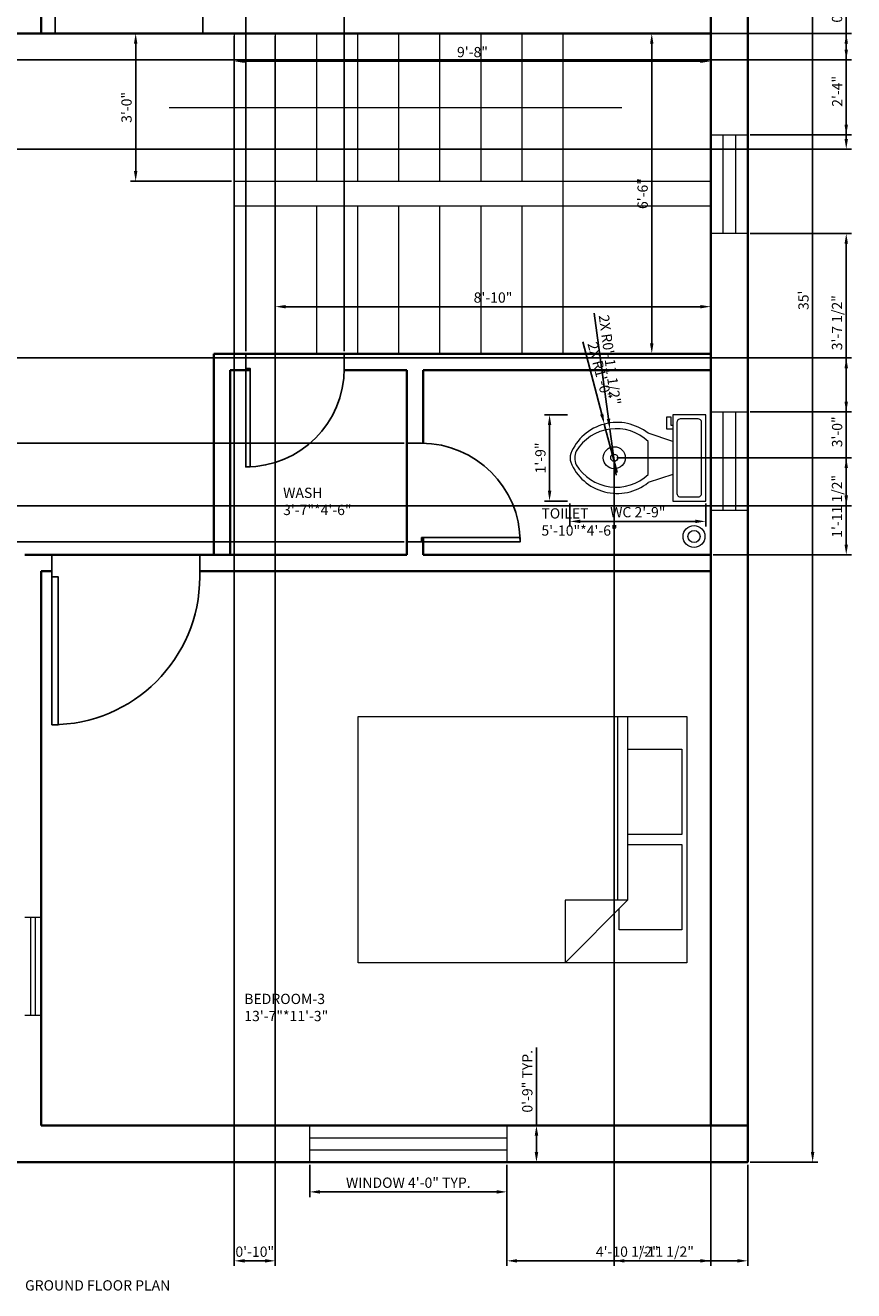
# Model space of a CAD drawing. Units: inches. Extents: x 2655 to 3059, y 1617 to 2098.
# Tile 2 of 3: x 2857 to 3059, y 1617 to 1926. Entities that reach past the tile are written whole.
import ezdxf

# ---------------------------------------------------------------- set-up
doc = ezdxf.new("R2010")
doc.units = ezdxf.units.IN
for name, color, linetype, lineweight in [('A-ANNO-DIMS', 2, 'Continuous', 18), ('A-ANNO-TEXT', 7, 'Continuous', 18), ('A-AREA-IDEN', 7, 'Continuous', 18), ('A-DOOR', 3, 'Continuous', 25), ('A-FLOR-FIXT', 9, 'Continuous', 18), ('A-FLOR-STRS', 7, 'Continuous', 20), ('A-FURN', 8, 'Continuous', 18), ('A-GLAZ', 4, 'Continuous', 18), ('A-WALL', 7, 'Continuous', 35)]:
    doc.layers.add(name, color=color, linetype=linetype, lineweight=lineweight)
doc.styles.get("Standard").update_dxf_attribs({"font": 'arial.ttf'})
doc.dimstyles.new('ISO-25', dxfattribs={"dimtxt": 2.5, "dimasz": 2.5, "dimexe": 1.25, "dimexo": 0.625, "dimtad": 1, "dimdec": 1, "dimlunit": 3, "dimtxsty": 'Standard', "dimcen": 2.5, "dimadec": 0, "dimazin": 0, "dimtfac": 1, "dimtdec": 1, "dimtmove": 0, "dimatfit": 3, "dimfxl": 1, "dimarcsym": 0})

# ---------------------------------------------------------------- blocks, each defined once
blk = doc.blocks.new('*D1')
at = {"layer": 'A-ANNO-DIMS', "color": 0, "lineweight": -2, "transparency": 16777216}
for p, q in [((2907.77, 1923.14), (2907.77, 1915.77)), ((3023.77, 1923.14), (3023.77, 1915.77)), ((2910.27, 1917.02), (3021.27, 1917.02))]:
    blk.add_line(p, q, dxfattribs=at)
at = {"layer": 'A-ANNO-DIMS', "color": 0, "transparency": 16777216}
for points in [[(2910.27, 1917.43), (2910.27, 1916.6), (2907.77, 1917.02)], [(3021.27, 1917.43), (3021.27, 1916.6), (3023.77, 1917.02)]]:
    blk.add_solid(points, dxfattribs=at)
at = {"layer": 'Defpoints', "color": 0, "transparency": 16777216}
for p in [(2907.77, 1923.77), (3023.77, 1923.77), (3023.77, 1917.02)]:
    blk.add_point(p, dxfattribs=at)
at = {"layer": 'A-ANNO-DIMS', "color": 0, "transparency": 16777216, "insert": (2965.77, 1918.92), "char_height": 2.5, "attachment_point": 5}
blk.add_mtext('9\'-8"', dxfattribs=at)
blk = doc.blocks.new('*D2')
at = {"layer": 'A-ANNO-DIMS', "color": 0, "lineweight": -2, "transparency": 16777216}
for p, q in [((2917.77, 1846.39), (2917.77, 1858.47)), ((2920.27, 1857.22), (3021.27, 1857.22)), ((3023.77, 1846.39), (3023.77, 1858.47))]:
    blk.add_line(p, q, dxfattribs=at)
at = {"layer": 'A-ANNO-DIMS', "color": 0, "transparency": 16777216}
for points in [[(2920.27, 1857.63), (2920.27, 1856.8), (2917.77, 1857.22)], [(3021.27, 1857.63), (3021.27, 1856.8), (3023.77, 1857.22)]]:
    blk.add_solid(points, dxfattribs=at)
at = {"layer": 'Defpoints', "color": 0, "transparency": 16777216}
for p in [(3023.77, 1857.22), (2917.77, 1845.77), (3023.77, 1845.77)]:
    blk.add_point(p, dxfattribs=at)
at = {"layer": 'A-ANNO-DIMS', "color": 0, "transparency": 16777216, "insert": (2970.77, 1859.12), "char_height": 2.5, "attachment_point": 5}
blk.add_mtext('8\'-10"', dxfattribs=at)
blk = doc.blocks.new('*D3')
at = {"layer": 'A-ANNO-DIMS', "color": 0, "lineweight": -2, "transparency": 16777216}
for p, q in [((3023.14, 1923.77), (3008.17, 1923.77)), ((3009.42, 1921.27), (3009.42, 1848.27)), ((3023.14, 1845.77), (3008.17, 1845.77))]:
    blk.add_line(p, q, dxfattribs=at)
at = {"layer": 'A-ANNO-DIMS', "color": 0, "transparency": 16777216}
for points in [[(3009, 1921.27), (3009.84, 1921.27), (3009.42, 1923.77)], [(3009, 1848.27), (3009.84, 1848.27), (3009.42, 1845.77)]]:
    blk.add_solid(points, dxfattribs=at)
at = {"layer": 'Defpoints', "color": 0, "transparency": 16777216}
for p in [(3023.77, 1923.77), (3009.42, 1845.77), (3023.77, 1845.77)]:
    blk.add_point(p, dxfattribs=at)
at = {"layer": 'A-ANNO-DIMS', "color": 0, "transparency": 16777216, "insert": (3007.52, 1884.77), "char_height": 2.5, "attachment_point": 5, "rotation": 90}
blk.add_mtext('6\'-6"', dxfattribs=at)
blk = doc.blocks.new('*U5')
for p, q in [((0, 0), (0, -6)), ((40, 0), (40, -6))]:
    blk.add_line(p, q)
blk.add_lwpolyline([(0, 0), (0, 40), (1.75, 40), (1.75, 0)], close=True)
blk.add_arc((0, 0), 40, 0, 90)
blk = doc.blocks.new('Bed - Queen')
for p, q in [((0, -80.00003), (0, 0)), ((0, 0), (59.99999, 0)), ((59.99999, 0), (59.99999, -80.00003)), ((7.99999, -1.2), (28.79998, -1.2)), ((7.99999, -14.4), (7.99999, -1.2)), ((28.79998, -1.2), (28.79998, -14.4)), ((31.19999, -1.2), (51.99999, -1.2)), ((31.19999, -14.4), (31.19999, -1.2)), ((51.99999, -1.2), (51.99999, -16.4)), ((0, -14.4), (44.8, -14.4)), ((59.99999, -29.6), (44.8, -14.4)), ((44.8, -14.4), (44.8, -29.6)), ((44.8, -16.8), (0, -16.8)), ((51.99999, -16.4), (46.79936, -16.4)), ((44.8, -29.6), (59.99999, -29.6)), ((59.99999, -80.00003), (0, -80.00003))]:
    blk.add_line(p, q)
blk = doc.blocks.new('Toilet - top')
for p, q in [((9.5, -6), (9.5, -2)), ((-10, -8.5), (-8, -8.5)), ((-10, -9.5), (-10, -8.5)), ((-8, -8.5), (-8, -8)), ((-7, -8), (-7, -9.5)), ((-4, -8), (-6, -14)), ((4, -8), (6, -14)), ((-7, -9.5), (-10, -9.5)), ((4, -14), (-4, -14))]:
    blk.add_line(p, q)
blk.add_lwpolyline([(10.5, -8), (10.5, 0), (-10.5, 0), (-10.5, -8)], close=True)
for points in [[(-9.5, -2), (-9.5, -6)], [(8.5, -1), (-8.5, -1)], [(-8.5, -7), (8.5, -7)]]:
    blk.add_lwpolyline(points)
for centre, radius, start, end in [((-8.62, -1.88), 0.884, 81.8699, 188.1301), ((8.62, -1.88), 0.884, 351.8699, 98.1301), ((-8.62, -6.12), 0.884, 171.8699, 278.1301), ((8.62, -6.12), 0.884, 261.8699, 8.1301), ((3.52, -21.58), 12.17, 141.4691, 247.9714), ((4.2, -21.82), 11.33, 136.3677, 238.9468), ((-3.52, -21.58), 12.17, 292.0284, 38.5307), ((-4.2, -21.82), 11.33, 301.053, 43.6321), ((0, -27.88), 4, 245.7318, 294.2682), ((0, -29), 4, 254.8605, 285.1395)]:
    blk.add_arc(centre, radius, start, end)
blk = doc.blocks.new('*D10')
at = {"layer": 'A-ANNO-DIMS', "color": 0, "lineweight": -2, "transparency": 16777216}
for p, q in [((3033.39, 2068.77), (3049.84, 2068.77)), ((3048.59, 2066.27), (3048.59, 1651.27)), ((3033.39, 1648.77), (3049.84, 1648.77))]:
    blk.add_line(p, q, dxfattribs=at)
at = {"layer": 'A-ANNO-DIMS', "color": 0, "transparency": 16777216}
for points in [[(3048.17, 2066.27), (3049, 2066.27), (3048.59, 2068.77)], [(3048.17, 1651.27), (3049, 1651.27), (3048.59, 1648.77)]]:
    blk.add_solid(points, dxfattribs=at)
at = {"layer": 'Defpoints', "color": 0, "transparency": 16777216}
for p in [(3032.77, 2068.77), (3032.77, 1648.77), (3048.59, 1648.77)]:
    blk.add_point(p, dxfattribs=at)
at = {"layer": 'A-ANNO-DIMS', "color": 0, "transparency": 16777216, "insert": (3046.68, 1858.77), "char_height": 2.5, "attachment_point": 5, "rotation": 90}
blk.add_mtext("35'", dxfattribs=at)
blk = doc.blocks.new('WIN-48x9')
for p, q in [((0, 9), (48, 9)), ((0, 0), (0, 9)), ((48, 9), (48, 0)), ((0, 6), (48, 6)), ((48, 3), (0, 3)), ((48, 0), (0, 0))]:
    blk.add_line(p, q)
blk = doc.blocks.new('WIN-24x9')
for p, q in [((0, 0), (0, 24)), ((0, 24), (9, 24)), ((3, 0), (3, 24)), ((6, 24), (6, 0)), ((9, 24), (9, 0)), ((9, 0), (0, 0))]:
    blk.add_line(p, q)
blk = doc.blocks.new('*D13')
at = {"layer": 'A-ANNO-DIMS', "color": 0, "lineweight": -2, "transparency": 16777216}
for p, q in [((2926.15, 1648.14), (2926.15, 1640.32)), ((2974.15, 1648.14), (2974.15, 1640.32)), ((2928.65, 1641.57), (2971.65, 1641.57))]:
    blk.add_line(p, q, dxfattribs=at)
at = {"layer": 'A-ANNO-DIMS', "color": 0, "transparency": 16777216}
for points in [[(2928.65, 1641.98), (2928.65, 1641.15), (2926.15, 1641.57)], [(2971.65, 1641.98), (2971.65, 1641.15), (2974.15, 1641.57)]]:
    blk.add_solid(points, dxfattribs=at)
at = {"layer": 'Defpoints', "color": 0, "transparency": 16777216}
for p in [(2926.15, 1648.77), (2974.15, 1648.77), (2974.15, 1641.57)]:
    blk.add_point(p, dxfattribs=at)
at = {"layer": 'A-ANNO-DIMS', "color": 0, "transparency": 16777216, "insert": (2950.15, 1643.48), "char_height": 2.5, "attachment_point": 5}
blk.add_mtext('WINDOW 4\'-0" TYP.', dxfattribs=at)
blk = doc.blocks.new('*D14')
at = {"layer": 'A-ANNO-DIMS', "color": 0, "lineweight": -2, "transparency": 16777216}
for p, q in [((2981.35, 1657.77), (2981.35, 1676.76)), ((2974.78, 1657.77), (2982.6, 1657.77)), ((2981.35, 1651.27), (2981.35, 1655.27)), ((2974.78, 1648.77), (2982.6, 1648.77))]:
    blk.add_line(p, q, dxfattribs=at)
at = {"layer": 'A-ANNO-DIMS', "color": 0, "transparency": 16777216}
for points in [[(2980.93, 1655.27), (2981.77, 1655.27), (2981.35, 1657.77)], [(2980.93, 1651.27), (2981.77, 1651.27), (2981.35, 1648.77)]]:
    blk.add_solid(points, dxfattribs=at)
at = {"layer": 'Defpoints', "color": 0, "transparency": 16777216}
for p in [(2974.15, 1657.77), (2981.35, 1657.77), (2974.15, 1648.77)]:
    blk.add_point(p, dxfattribs=at)
at = {"layer": 'A-ANNO-DIMS', "color": 0, "transparency": 16777216, "insert": (2979.45, 1668.51), "char_height": 2.5, "attachment_point": 5, "rotation": 90}
blk.add_mtext('0\'-9" TYP.', dxfattribs=at)
blk = doc.blocks.new('*D19')
at = {"layer": 'A-ANNO-DIMS', "color": 0, "lineweight": -2, "transparency": 16777216}
for p, q in [((2989.5, 1809.25), (2989.5, 1803.66)), ((3022.55, 1809.25), (3022.55, 1803.66)), ((2992, 1804.91), (3020.05, 1804.91))]:
    blk.add_line(p, q, dxfattribs=at)
at = {"layer": 'A-ANNO-DIMS', "color": 0, "transparency": 16777216}
for points in [[(2992, 1805.33), (2992, 1804.5), (2989.5, 1804.91)], [(3020.05, 1805.33), (3020.05, 1804.5), (3022.55, 1804.91)]]:
    blk.add_solid(points, dxfattribs=at)
at = {"layer": 'Defpoints', "color": 0, "transparency": 16777216}
for p in [(2989.5, 1809.87), (3022.55, 1809.87), (3022.55, 1804.91)]:
    blk.add_point(p, dxfattribs=at)
at = {"layer": 'A-ANNO-DIMS', "color": 0, "transparency": 16777216, "insert": (3006.02, 1806.83), "char_height": 2.5, "attachment_point": 5}
blk.add_mtext('WC 2\'-9"', dxfattribs=at)
blk = doc.blocks.new('*D20')
at = {"layer": 'A-ANNO-DIMS', "color": 0, "lineweight": -2, "transparency": 16777216}
for p, q in [((2988.88, 1830.87), (2983.29, 1830.87)), ((2984.54, 1828.37), (2984.54, 1812.37)), ((2988.88, 1809.87), (2983.29, 1809.87))]:
    blk.add_line(p, q, dxfattribs=at)
at = {"layer": 'A-ANNO-DIMS', "color": 0, "transparency": 16777216}
for points in [[(2984.13, 1828.37), (2984.96, 1828.37), (2984.54, 1830.87)], [(2984.13, 1812.37), (2984.96, 1812.37), (2984.54, 1809.87)]]:
    blk.add_solid(points, dxfattribs=at)
at = {"layer": 'Defpoints', "color": 0, "transparency": 16777216}
for p in [(2989.5, 1830.87), (2984.54, 1809.87), (2989.5, 1809.87)]:
    blk.add_point(p, dxfattribs=at)
at = {"layer": 'A-ANNO-DIMS', "color": 0, "transparency": 16777216, "insert": (2982.64, 1820.37), "char_height": 2.5, "attachment_point": 5, "rotation": 90}
blk.add_mtext('1\'-9"', dxfattribs=at)
blk = doc.blocks.new('*D27')
at = {"layer": 'A-ANNO-DIMS', "color": 0, "lineweight": -2, "transparency": 16777216}
for p, q in [((3033.39, 1985.21), (3058.02, 1985.21)), ((3056.77, 1982.71), (3056.77, 1901.56)), ((3033.39, 1899.06), (3058.02, 1899.06))]:
    blk.add_line(p, q, dxfattribs=at)
at = {"layer": 'A-ANNO-DIMS', "color": 0, "transparency": 16777216}
for points in [[(3056.35, 1982.71), (3057.19, 1982.71), (3056.77, 1985.21)], [(3056.35, 1901.56), (3057.19, 1901.56), (3056.77, 1899.06)]]:
    blk.add_solid(points, dxfattribs=at)
at = {"layer": 'Defpoints', "color": 0, "transparency": 16777216}
for p in [(3032.77, 1985.21), (3032.77, 1899.06), (3056.77, 1899.06)]:
    blk.add_point(p, dxfattribs=at)
at = {"layer": 'A-ANNO-DIMS', "color": 0, "transparency": 16777216, "insert": (3054.89, 1942.13), "char_height": 2.5, "attachment_point": 5, "rotation": 90}
blk.add_mtext('7\'-2"', dxfattribs=at)
blk = doc.blocks.new('*D28')
at = {"layer": 'A-ANNO-DIMS', "color": 0, "lineweight": -2, "transparency": 16777216}
for p, q in [((3033.39, 1875.06), (3058.02, 1875.06)), ((3056.77, 1872.56), (3056.77, 1834.08)), ((3033.39, 1831.58), (3058.02, 1831.58))]:
    blk.add_line(p, q, dxfattribs=at)
at = {"layer": 'A-ANNO-DIMS', "color": 0, "transparency": 16777216}
for points in [[(3056.35, 1872.56), (3057.19, 1872.56), (3056.77, 1875.06)], [(3056.35, 1834.08), (3057.19, 1834.08), (3056.77, 1831.58)]]:
    blk.add_solid(points, dxfattribs=at)
at = {"layer": 'Defpoints', "color": 0, "transparency": 16777216}
for p in [(3032.77, 1875.06), (3032.77, 1831.58), (3056.77, 1831.58)]:
    blk.add_point(p, dxfattribs=at)
at = {"layer": 'A-ANNO-DIMS', "color": 0, "transparency": 16777216, "insert": (3054.85, 1853.32), "char_height": 2.5, "attachment_point": 5, "rotation": 90}
blk.add_mtext('3\'-7 1/2"', dxfattribs=at)
blk = doc.blocks.new('*D29')
at = {"layer": 'A-ANNO-DIMS', "color": 0, "lineweight": -2, "transparency": 16777216}
for p, q in [((2974.15, 1648.14), (2974.15, 1623.52)), ((3032.77, 1648.14), (3032.77, 1623.52)), ((3030.27, 1624.77), (2976.65, 1624.77))]:
    blk.add_line(p, q, dxfattribs=at)
at = {"layer": 'A-ANNO-DIMS', "color": 0, "transparency": 16777216}
for points in [[(2976.65, 1625.18), (2976.65, 1624.35), (2974.15, 1624.77)], [(3030.27, 1625.18), (3030.27, 1624.35), (3032.77, 1624.77)]]:
    blk.add_solid(points, dxfattribs=at)
at = {"layer": 'Defpoints', "color": 0, "transparency": 16777216}
for p in [(2974.15, 1648.77), (3032.77, 1648.77), (2974.15, 1624.77)]:
    blk.add_point(p, dxfattribs=at)
at = {"layer": 'A-ANNO-DIMS', "color": 0, "transparency": 16777216, "insert": (3003.46, 1626.68), "char_height": 2.5, "attachment_point": 5}
blk.add_mtext('4\'-10 1/2"', dxfattribs=at)
blk = doc.blocks.new('*D37')
at = {"layer": 'A-ANNO-DIMS', "color": 0, "lineweight": -2, "transparency": 16777216}
for p, q in [((2907.77, 1923.14), (2907.77, 1623.52)), ((2917.77, 1923.14), (2917.77, 1623.52)), ((2910.27, 1624.77), (2915.27, 1624.77))]:
    blk.add_line(p, q, dxfattribs=at)
at = {"layer": 'A-ANNO-DIMS', "color": 0, "transparency": 16777216}
for points in [[(2910.27, 1625.18), (2910.27, 1624.35), (2907.77, 1624.77)], [(2915.27, 1625.18), (2915.27, 1624.35), (2917.77, 1624.77)]]:
    blk.add_solid(points, dxfattribs=at)
at = {"layer": 'Defpoints', "color": 0, "transparency": 16777216}
for p in [(2907.77, 1923.77), (2917.77, 1923.77), (2917.77, 1624.77)]:
    blk.add_point(p, dxfattribs=at)
at = {"layer": 'A-ANNO-DIMS', "color": 0, "transparency": 16777216, "insert": (2912.77, 1626.67), "char_height": 2.5, "attachment_point": 5}
blk.add_mtext('0\'-10"', dxfattribs=at)
blk = doc.blocks.new('*D38')
at = {"layer": 'A-ANNO-DIMS', "color": 0, "lineweight": -2, "transparency": 16777216}
for p, q in [((2907.14, 1923.77), (2882.52, 1923.77)), ((2883.77, 1890.27), (2883.77, 1921.27)), ((2907.14, 1887.77), (2882.52, 1887.77))]:
    blk.add_line(p, q, dxfattribs=at)
at = {"layer": 'A-ANNO-DIMS', "color": 0, "transparency": 16777216}
for points in [[(2883.35, 1921.27), (2884.19, 1921.27), (2883.77, 1923.77)], [(2883.35, 1890.27), (2884.19, 1890.27), (2883.77, 1887.77)]]:
    blk.add_solid(points, dxfattribs=at)
at = {"layer": 'Defpoints', "color": 0, "transparency": 16777216}
for p in [(2883.77, 1923.77), (2907.77, 1923.77), (2907.77, 1887.77)]:
    blk.add_point(p, dxfattribs=at)
at = {"layer": 'A-ANNO-DIMS', "color": 0, "transparency": 16777216, "insert": (2881.87, 1905.77), "char_height": 2.5, "attachment_point": 5, "rotation": 90}
blk.add_mtext('3\'-0"', dxfattribs=at)
blk = doc.blocks.new('*D39')
at = {"layer": 'A-ANNO-DIMS', "color": 0, "lineweight": -2, "transparency": 16777216}
for p, q in [((2910.57, 1846.39), (2910.57, 2094.02)), ((2934.57, 1846.39), (2934.57, 2094.02)), ((2913.07, 2092.77), (2932.07, 2092.77))]:
    blk.add_line(p, q, dxfattribs=at)
at = {"layer": 'A-ANNO-DIMS', "color": 0, "transparency": 16777216}
for points in [[(2913.07, 2093.18), (2913.07, 2092.35), (2910.57, 2092.77)], [(2932.07, 2093.18), (2932.07, 2092.35), (2934.57, 2092.77)]]:
    blk.add_solid(points, dxfattribs=at)
at = {"layer": 'Defpoints', "color": 0, "transparency": 16777216}
for p in [(2934.57, 2092.77), (2910.57, 1845.77), (2934.57, 1845.77)]:
    blk.add_point(p, dxfattribs=at)
at = {"layer": 'A-ANNO-DIMS', "color": 0, "transparency": 16777216, "insert": (2922.57, 2094.67), "char_height": 2.5, "attachment_point": 5}
blk.add_mtext('2\'-0"', dxfattribs=at)
blk = doc.blocks.new('*D40')
at = {"layer": 'A-ANNO-DIMS', "color": 0, "lineweight": -2, "transparency": 16777216}
for p, q in [((2949.14, 1823.93), (2659.52, 1823.93)), ((2660.77, 1802.43), (2660.77, 1821.43)), ((2949.14, 1799.93), (2659.52, 1799.93))]:
    blk.add_line(p, q, dxfattribs=at)
at = {"layer": 'A-ANNO-DIMS', "color": 0, "transparency": 16777216}
for points in [[(2660.35, 1821.43), (2661.19, 1821.43), (2660.77, 1823.93)], [(2660.35, 1802.43), (2661.19, 1802.43), (2660.77, 1799.93)]]:
    blk.add_solid(points, dxfattribs=at)
at = {"layer": 'Defpoints', "color": 0, "transparency": 16777216}
for p in [(2660.77, 1823.93), (2949.77, 1823.93), (2949.77, 1799.93)]:
    blk.add_point(p, dxfattribs=at)
at = {"layer": 'A-ANNO-DIMS', "color": 0, "transparency": 16777216, "insert": (2658.87, 1811.93), "char_height": 2.5, "attachment_point": 5, "rotation": 90}
blk.add_mtext('2\'-0"', dxfattribs=at)
blk = doc.blocks.new('*D41')
at = {"layer": 'A-ANNO-DIMS', "color": 0, "lineweight": -2, "transparency": 16777216}
for p, q in [((3000.28, 1819.77), (3000.28, 1623.52)), ((3023.77, 1796.14), (3023.77, 1623.52)), ((3021.27, 1624.77), (3002.78, 1624.77))]:
    blk.add_line(p, q, dxfattribs=at)
at = {"layer": 'A-ANNO-DIMS', "color": 0, "transparency": 16777216}
for points in [[(3002.78, 1625.18), (3002.78, 1624.35), (3000.28, 1624.77)], [(3021.27, 1625.18), (3021.27, 1624.35), (3023.77, 1624.77)]]:
    blk.add_solid(points, dxfattribs=at)
at = {"layer": 'Defpoints', "color": 0, "transparency": 16777216}
for p in [(3000.28, 1820.4), (3023.77, 1796.77), (3000.28, 1624.77)]:
    blk.add_point(p, dxfattribs=at)
at = {"layer": 'A-ANNO-DIMS', "color": 0, "transparency": 16777216, "insert": (3012.03, 1626.68), "char_height": 2.5, "attachment_point": 5}
blk.add_mtext('1\'-11 1/2"', dxfattribs=at)
blk = doc.blocks.new('*D42')
at = {"layer": 'A-ANNO-DIMS', "color": 0, "lineweight": -2, "transparency": 16777216}
for p, q in [((3000.91, 1820.4), (3058.02, 1820.4)), ((3056.77, 1799.27), (3056.77, 1817.9)), ((3024.39, 1796.77), (3058.02, 1796.77))]:
    blk.add_line(p, q, dxfattribs=at)
at = {"layer": 'A-ANNO-DIMS', "color": 0, "transparency": 16777216}
for points in [[(3056.35, 1817.9), (3057.19, 1817.9), (3056.77, 1820.4)], [(3056.35, 1799.27), (3057.19, 1799.27), (3056.77, 1796.77)]]:
    blk.add_solid(points, dxfattribs=at)
at = {"layer": 'Defpoints', "color": 0, "transparency": 16777216}
for p in [(3000.28, 1820.4), (3056.77, 1820.4), (3023.77, 1796.77)]:
    blk.add_point(p, dxfattribs=at)
at = {"layer": 'A-ANNO-DIMS', "color": 0, "transparency": 16777216, "insert": (3054.85, 1808.58), "char_height": 2.5, "attachment_point": 5, "rotation": 90}
blk.add_mtext('1\'-11 1/2"', dxfattribs=at)
blk = doc.blocks.new('*D44')
at = {"layer": 'A-ANNO-DIMS', "color": 0, "lineweight": -2, "transparency": 16777216}
for p, q in [((2766.39, 1923.77), (3058.02, 1923.77)), ((3056.77, 1898.09), (3056.77, 1921.27)), ((2766.39, 1895.59), (3058.02, 1895.59))]:
    blk.add_line(p, q, dxfattribs=at)
at = {"layer": 'A-ANNO-DIMS', "color": 0, "transparency": 16777216}
for points in [[(3056.35, 1921.27), (3057.19, 1921.27), (3056.77, 1923.77)], [(3056.35, 1898.09), (3057.19, 1898.09), (3056.77, 1895.59)]]:
    blk.add_solid(points, dxfattribs=at)
at = {"layer": 'Defpoints', "color": 0, "transparency": 16777216}
for p in [(2765.77, 1923.77), (3056.77, 1923.77), (2765.77, 1895.59)]:
    blk.add_point(p, dxfattribs=at)
at = {"layer": 'A-ANNO-DIMS', "color": 0, "transparency": 16777216, "insert": (3054.89, 1909.68), "char_height": 2.5, "attachment_point": 5, "rotation": 90}
blk.add_mtext('2\'-4"', dxfattribs=at)
blk = doc.blocks.new('*D45')
at = {"layer": 'A-ANNO-DIMS', "color": 0, "lineweight": -2, "transparency": 16777216}
for p, q in [((2770.39, 1844.73), (3058.02, 1844.73)), ((3056.77, 1811.23), (3056.77, 1842.23)), ((2770.39, 1808.73), (3058.02, 1808.73))]:
    blk.add_line(p, q, dxfattribs=at)
at = {"layer": 'A-ANNO-DIMS', "color": 0, "transparency": 16777216}
for points in [[(3056.35, 1842.23), (3057.19, 1842.23), (3056.77, 1844.73)], [(3056.35, 1811.23), (3057.19, 1811.23), (3056.77, 1808.73)]]:
    blk.add_solid(points, dxfattribs=at)
at = {"layer": 'Defpoints', "color": 0, "transparency": 16777216}
for p in [(2769.77, 1844.73), (3056.77, 1844.73), (2769.77, 1808.73)]:
    blk.add_point(p, dxfattribs=at)
at = {"layer": 'A-ANNO-DIMS', "color": 0, "transparency": 16777216, "insert": (3054.87, 1826.73), "char_height": 2.5, "attachment_point": 5, "rotation": 90}
blk.add_mtext('3\'-0"', dxfattribs=at)
blk = doc.blocks.new('*D50')
at = {"layer": 'A-ANNO-DIMS', "color": 0, "lineweight": -2, "transparency": 16777216}
for p, q in [((3056.77, 1923.77), (3056.77, 1939.99)), ((2766.39, 1923.77), (3058.02, 1923.77)), ((3056.77, 1919.87), (3056.77, 1921.27)), ((2751.1, 1917.37), (3058.02, 1917.37))]:
    blk.add_line(p, q, dxfattribs=at)
at = {"layer": 'A-ANNO-DIMS', "color": 0, "transparency": 16777216}
for points in [[(3056.35, 1921.27), (3057.19, 1921.27), (3056.77, 1923.77)], [(3056.35, 1919.87), (3057.19, 1919.87), (3056.77, 1917.37)]]:
    blk.add_solid(points, dxfattribs=at)
at = {"layer": 'Defpoints', "color": 0, "transparency": 16777216}
for p in [(2765.77, 1923.77), (3056.77, 1923.77), (2750.48, 1917.37)]:
    blk.add_point(p, dxfattribs=at)
at = {"layer": 'A-ANNO-DIMS', "color": 0, "transparency": 16777216, "insert": (3054.85, 1933.13), "char_height": 2.5, "attachment_point": 5, "rotation": 90}
blk.add_mtext('0\'-6 1/2"', dxfattribs=at)
blk = doc.blocks.new('*D52')
at = {"layer": 'A-ANNO-DIMS', "color": 0, "lineweight": -2, "transparency": 16777216}
for p, q in [((2992.61, 1848.64), (2997.24, 1831.04)), ((3000.97, 1816.85), (2997.87, 1828.62))]:
    blk.add_line(p, q, dxfattribs=at)
at = {"layer": 'A-ANNO-DIMS', "color": 0, "transparency": 16777216}
blk.add_solid([(2997.64, 1831.14), (2996.84, 1830.93), (2997.87, 1828.62)], dxfattribs=at)
at = {"layer": 'Defpoints', "color": 0, "transparency": 16777216}
for p in [(2997.87, 1828.62), (3000.97, 1816.85)]:
    blk.add_point(p, dxfattribs=at)
at = {"layer": 'A-ANNO-DIMS', "color": 0, "transparency": 16777216, "insert": (2996.45, 1841.53), "char_height": 2.5, "attachment_point": 5, "rotation": 284.7221}
blk.add_mtext('2X R1\'-0"', dxfattribs=at)
blk = doc.blocks.new('*D53')
at = {"layer": 'A-ANNO-DIMS', "color": 0, "lineweight": -2, "transparency": 16777216}
for p, q in [((2995.43, 1855.61), (2998.89, 1829.88)), ((3000.73, 1816.17), (2999.22, 1827.4))]:
    blk.add_line(p, q, dxfattribs=at)
at = {"layer": 'A-ANNO-DIMS', "color": 0, "transparency": 16777216}
blk.add_solid([(2999.3, 1829.93), (2998.47, 1829.82), (2999.22, 1827.4)], dxfattribs=at)
at = {"layer": 'Defpoints', "color": 0, "transparency": 16777216}
for p in [(2999.22, 1827.4), (3000.73, 1816.17)]:
    blk.add_point(p, dxfattribs=at)
at = {"layer": 'A-ANNO-DIMS', "color": 0, "transparency": 16777216, "insert": (2998.89, 1844.24), "char_height": 2.5, "attachment_point": 5, "rotation": 277.6576}
blk.add_mtext('2X R0\'-11 1/2"', dxfattribs=at)

msp = doc.modelspace()

# ---------------------------------------------------------------- linework, layer by layer
at = {"layer": 'A-FLOR-FIXT'}
for centre, radius in [((3000.28, 1820.4), 2.69), ((3000.28, 1820.4), 0.863), ((3019.71, 1801.24), 2.66), ((3019.71, 1801.24), 1.47)]:
    msp.add_circle(centre, radius, dxfattribs=at)
at = {"layer": 'A-FLOR-STRS'}
for p, q in [((2907.77, 1923.77), (2907.77, 1881.77)), ((2917.77, 1923.77), (2917.77, 1887.77)), ((2927.77, 1923.77), (2927.77, 1887.77)), ((2937.77, 1923.77), (2937.77, 1887.77)), ((2947.77, 1923.77), (2947.77, 1887.77)), ((2957.77, 1923.77), (2957.77, 1887.77)), ((2967.77, 1923.77), (2967.77, 1887.77)), ((2977.77, 1923.77), (2977.77, 1887.77)), ((2987.77, 1923.77), (2987.77, 1845.77)), ((2891.94, 1905.77), (3002.15, 1905.77)), ((2907.77, 1887.77), (3023.77, 1887.77)), ((2907.77, 1881.77), (3023.77, 1881.77)), ((2917.77, 1881.77), (2917.77, 1845.77)), ((2927.77, 1881.77), (2927.77, 1845.77)), ((2937.77, 1881.77), (2937.77, 1845.77)), ((2947.77, 1881.77), (2947.77, 1845.77)), ((2957.77, 1881.77), (2957.77, 1845.77)), ((2967.77, 1881.77), (2967.77, 1845.77)), ((2977.77, 1881.77), (2977.77, 1845.77))]:
    msp.add_line(p, q, dxfattribs=at)
at = {"layer": 'A-GLAZ'}
for p, q in [((2856.77, 1708.5), (2860.77, 1708.5)), ((2858.27, 1684.5), (2858.27, 1708.5)), ((2859.27, 1708.5), (2859.27, 1684.5)), ((2860.77, 1708.5), (2860.77, 1684.5)), ((2860.77, 1684.5), (2856.77, 1684.5))]:
    msp.add_line(p, q, dxfattribs=at)
at = {"layer": 'A-WALL'}
for p, q in [((3032.77, 2068.77), (3032.77, 1648.77)), ((2860.77, 2059.77), (2860.77, 1923.77)), ((2860.77, 1923.77), (2860.77, 2059.77)), ((3023.77, 2059.77), (3023.77, 1657.77)), ((2769.77, 1923.77), (3023.77, 1923.77)), ((2902.77, 1845.77), (3023.77, 1845.77)), ((2902.77, 1845.77), (2902.77, 1796.77)), ((2906.77, 1841.77), (2911.62, 1841.77)), ((2906.77, 1841.77), (2906.77, 1796.77)), ((2934.57, 1841.77), (2949.77, 1841.77)), ((2949.77, 1841.77), (2949.77, 1796.77)), ((2953.77, 1841.77), (2953.77, 1823.93)), ((2953.77, 1841.77), (3023.77, 1841.77)), ((2953.77, 1800.98), (2953.77, 1796.77)), ((2949.77, 1796.77), (2856.77, 1796.77)), ((3023.77, 1796.77), (2953.77, 1796.77)), ((2860.77, 1657.77), (2860.77, 1792.77)), ((2863.36, 1792.77), (2860.77, 1792.77)), ((3023.77, 1792.77), (2899.36, 1792.77)), ((3032.77, 1657.77), (2860.77, 1657.77)), ((3032.77, 1648.77), (2684.77, 1648.77))]:
    msp.add_line(p, q, dxfattribs=at)

# ---------------------------------------------------------------- block references
at = {"layer": 'A-DOOR', "xscale": 0.9, "yscale": 0.9, "zscale": 0.9}
msp.add_blockref('*U5', (2864.13, 1929.17), dxfattribs=at)
at = {"layer": 'A-DOOR'}
for p, xscale, yscale, zscale, rotation in [((2910.57, 1842.17), -0.6, 0.6, 0.6, 180), ((2953.37, 1799.93), -0.6, 0.6, 0.6, 270), ((2863.36, 1791.37), -0.9, 0.9, 0.9, 180)]:
    msp.add_blockref('*U5', p, dxfattribs=dict(at, xscale=xscale, yscale=yscale, zscale=zscale, rotation=rotation))
at = {"layer": 'A-FLOR-FIXT', "rotation": 270}
msp.add_blockref('Toilet - top', (3022.55, 1820.37), dxfattribs=at)
at = {"layer": 'A-FURN', "rotation": 270}
msp.add_blockref('Bed - Queen', (3017.92, 1757.4), dxfattribs=at)
at = {"layer": 'A-GLAZ'}
for name, p in [('WIN-24x9', (3023.77, 1875.06)), ('WIN-24x9', (3023.77, 1807.58)), ('WIN-48x9', (2926.15, 1648.77))]:
    msp.add_blockref(name, p, dxfattribs=at)

# ---------------------------------------------------------------- texts
at = {"layer": 'A-ANNO-TEXT', "insert": (2856.84, 1620.04), "char_height": 2.5, "attachment_point": 1}
msp.add_mtext_dynamic_manual_height_columns('GROUND FLOOR PLAN', width=304.6086, gutter_width=12.5, heights=[0], dxfattribs=at)
at = {"layer": 'A-AREA-IDEN', "char_height": 2.5, "attachment_point": 1}
for s, width, insert in [('WASH\\P3\'-7"*4\'-6"', 24.9975, (2919.67, 1813.12)), ('TOILET\\P5\'-10"*4\'-6"', 20.0514, (2982.56, 1808.11)), ('BEDROOM-3\\P13\'-7"*11\'-3"', 65.1514, (2910.21, 1689.83))]:
    msp.add_mtext_dynamic_manual_height_columns(s, width=width, gutter_width=12.5, heights=[0], dxfattribs=dict(at, insert=insert))

# ---------------------------------------------------------------- dimensions: what is measured, and where the dimension line sits
at = {"layer": 'A-ANNO-DIMS'}
for base, p1, p2, override, picture, middle in [((2934.57, 2092.77), (2910.57, 1845.77), (2934.57, 1845.77), {"dimdec": 1, "dimlfac": 1, "dimrnd": 0, "dimzin": 1, "dimdsep": 46, "dimlunit": 4, "dimfrac": 2}, '*D39', (2922.57, 2094.67)), ((3023.77, 1917.02), (2907.77, 1923.77), (3023.77, 1923.77), {"dimclrd": 0, "dimclre": 0, "dimclrt": 0}, '*D1', (2965.77, 1918.92)), ((2917.77, 1624.77), (2907.77, 1923.77), (2917.77, 1923.77), {"dimdec": 1, "dimlfac": 1, "dimrnd": 0, "dimzin": 1, "dimdsep": 46, "dimlunit": 4, "dimfrac": 2}, '*D37', (2912.77, 1626.67)), ((3023.77, 1857.22), (2917.77, 1845.77), (3023.77, 1845.77), {"dimclrd": 0, "dimclre": 0, "dimclrt": 0}, '*D2', (2970.77, 1859.12)), ((3000.28, 1624.77), (3023.77, 1796.77), (3000.28, 1820.4), {"dimdec": 1, "dimlfac": 1, "dimrnd": 0, "dimzin": 1, "dimdsep": 46, "dimlunit": 4, "dimfrac": 2}, '*D41', (3012.03, 1626.68)), ((2974.15, 1624.77), (3032.77, 1648.77), (2974.15, 1648.77), {"dimdec": 1, "dimlfac": 1, "dimrnd": 0, "dimzin": 1, "dimdsep": 46, "dimlunit": 4, "dimfrac": 2}, '*D29', (3003.46, 1626.68))]:
    dim = msp.add_linear_dim(base=base, p1=p1, p2=p2, dimstyle='ISO-25', override=override, dxfattribs=at)
    dim.commit()
    dim.dimension.update_dxf_attribs({"geometry": picture, "text_midpoint": middle})
for base, p1, p2, angle, override, picture, middle in [((3048.59, 1648.77), (3032.77, 2068.77), (3032.77, 1648.77), 90, {"dimclrd": 0, "dimclre": 0, "dimclrt": 0}, '*D10', (3046.68, 1858.77)), ((3056.7686, 1899.0573), (3032.7686, 1985.2098), (3032.7677, 1899.0573), 90, {"dimdec": 1, "dimlfac": 1, "dimrnd": 0, "dimzin": 1, "dimdsep": 46, "dimlunit": 4, "dimfrac": 2}, '*D27', (3054.8885, 1942.1335)), ((3056.77, 1923.77), (2750.48, 1917.37), (2765.77, 1923.77), 90, {"dimdec": 1, "dimlfac": 1, "dimrnd": 0, "dimzin": 1, "dimdsep": 46, "dimlunit": 4, "dimfrac": 2}, '*D50', (3054.85, 1933.13)), ((3056.77, 1923.77), (2765.77, 1895.59), (2765.77, 1923.77), 90, {"dimdec": 1, "dimlfac": 1, "dimrnd": 0, "dimzin": 1, "dimdsep": 46, "dimlunit": 4, "dimfrac": 2}, '*D44', (3054.89, 1909.68)), ((2883.77, 1923.77), (2907.77, 1887.77), (2907.77, 1923.77), 90, {"dimdec": 1, "dimlfac": 1, "dimrnd": 0, "dimzin": 1, "dimdsep": 46, "dimlunit": 4, "dimfrac": 2}, '*D38', (2881.87, 1905.77)), ((3009.42, 1845.77), (3023.77, 1923.77), (3023.77, 1845.77), 90, {"dimclrd": 0, "dimclre": 0, "dimclrt": 0}, '*D3', (3007.52, 1884.77)), ((3056.77, 1831.58), (3032.77, 1875.06), (3032.77, 1831.58), 90, {"dimdec": 1, "dimlfac": 1, "dimrnd": 0, "dimzin": 1, "dimdsep": 46, "dimlunit": 4, "dimfrac": 2}, '*D28', (3054.85, 1853.32)), ((3056.77, 1844.73), (2769.77, 1808.73), (2769.77, 1844.73), 90, {"dimdec": 1, "dimlfac": 1, "dimrnd": 0, "dimzin": 1, "dimdsep": 46, "dimlunit": 4, "dimfrac": 2}, '*D45', (3054.87, 1826.73)), ((2984.54, 1809.87), (2989.5, 1830.87), (2989.5, 1809.87), 270, {"dimdec": 1, "dimlfac": 1, "dimrnd": 0, "dimzin": 1, "dimdsep": 46, "dimlunit": 4, "dimfrac": 2}, '*D20', (2982.64, 1820.37)), ((2660.77, 1823.93), (2949.77, 1799.93), (2949.77, 1823.93), 90, {"dimdec": 1, "dimlfac": 1, "dimrnd": 0, "dimzin": 1, "dimdsep": 46, "dimlunit": 4, "dimfrac": 2}, '*D40', (2658.87, 1811.93)), ((3056.77, 1820.4), (3023.77, 1796.77), (3000.28, 1820.4), 90, {"dimdec": 1, "dimlfac": 1, "dimrnd": 0, "dimzin": 1, "dimdsep": 46, "dimlunit": 4, "dimfrac": 2}, '*D42', (3054.85, 1808.58))]:
    dim = msp.add_linear_dim(base=base, p1=p1, p2=p2, angle=angle, dimstyle='ISO-25', override=override, dxfattribs=at)
    dim.commit()
    dim.dimension.update_dxf_attribs({"geometry": picture, "text_midpoint": middle})
for center, mpoint, picture, middle in [((3000.73, 1816.17), (2999.22, 1827.4), '*D53', (2998.89, 1844.24)), ((3000.97, 1816.85), (2997.87, 1828.62), '*D52', (2996.45, 1841.53))]:
    dim = msp.add_radius_dim(center=center, mpoint=mpoint, text='2X <>', dimstyle='ISO-25', override={"dimdec": 1, "dimlfac": 1, "dimrnd": 0, "dimzin": 1, "dimdsep": 46, "dimlunit": 4, "dimfrac": 2}, dxfattribs=at)
    dim.commit()
    dim.dimension.update_dxf_attribs({"geometry": picture, "text_midpoint": middle})
for base, p1, p2, text, picture, middle in [((3022.547, 1804.9132), (2989.5008, 1809.8701), (3022.547, 1809.8701), 'WC <>', '*D19', (3006.0239, 1806.8308)), ((2974.15, 1641.57), (2926.15, 1648.77), (2974.15, 1648.77), 'WINDOW <> TYP.', '*D13', (2950.15, 1643.48))]:
    dim = msp.add_linear_dim(base=base, p1=p1, p2=p2, text=text, dimstyle='ISO-25', override={"dimdec": 1, "dimlfac": 1, "dimrnd": 0, "dimzin": 1, "dimdsep": 46, "dimlunit": 4, "dimfrac": 2}, dxfattribs=at)
    dim.commit()
    dim.dimension.update_dxf_attribs({"geometry": picture, "text_midpoint": middle})
dim = msp.add_linear_dim(base=(2981.35, 1657.77), p1=(2974.15, 1648.77), p2=(2974.15, 1657.77), angle=90, text='<> TYP.', dimstyle='ISO-25', override={"dimdec": 1, "dimlfac": 1, "dimrnd": 0, "dimzin": 1, "dimdsep": 46, "dimlunit": 4, "dimfrac": 2}, dxfattribs=at)
dim.commit()
dim.dimension.update_dxf_attribs({"geometry": '*D14', "text_midpoint": (2979.45, 1668.51)})

doc.saveas('drawing.dxf')
